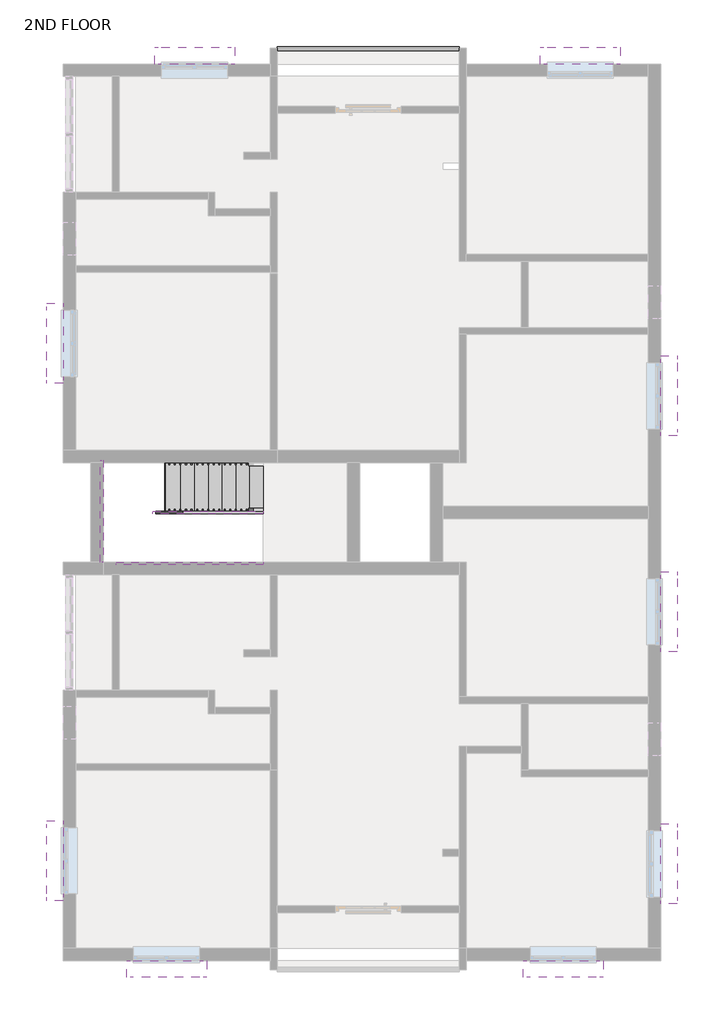
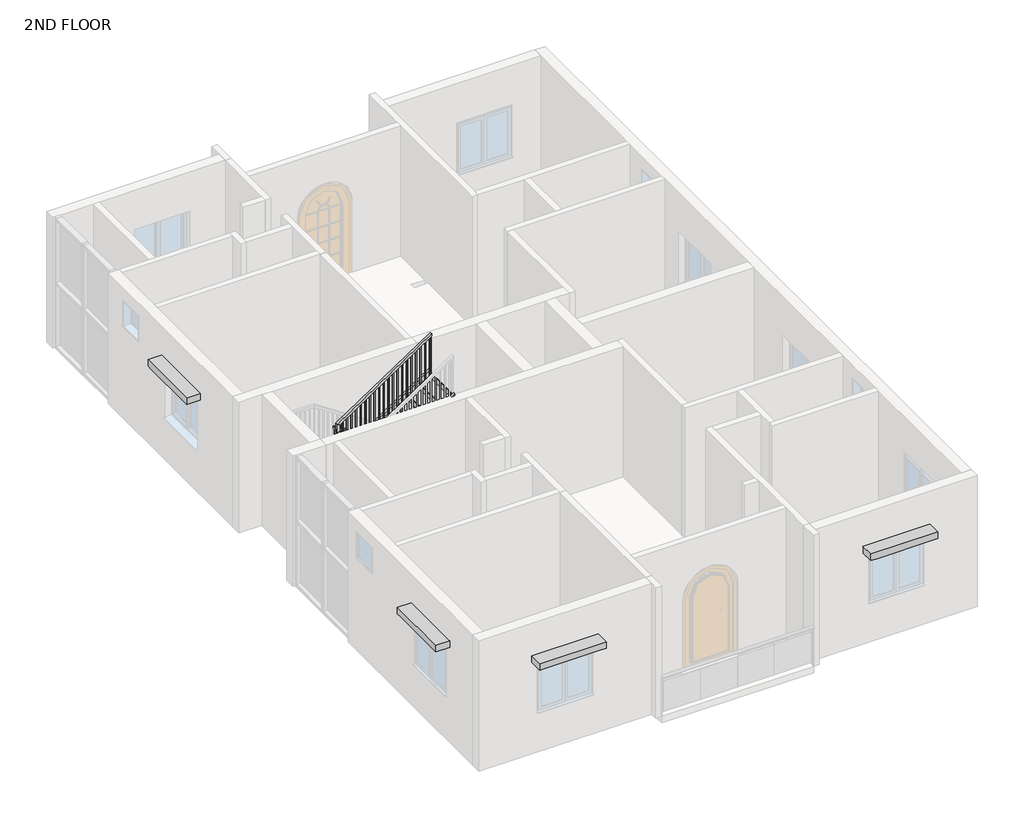
# One storey, part 4 of 4: 9 proxies, 5 members, 2 railings, 1 stair flight.
"""IFC4 building model written with IfcOpenShell, lengths in millimetres."""

from ifc_helpers import new_model, si_unit, point, frame, origin, place, context, project, spatial, polyline, ellipse_curve, trimmed, outline, extrude, faceted_brep, transform, mapped, element, save
from ifc_brep_helpers import plane_surface, extruded_surface, advanced_brep
from components import generic_models_11_generic_models_11_d301a5e8, generic_models_21_generic_models_21_87948dc1, generic_models_36_generic_models_36_9c63594f, generic_models_1_generic_models_1_fbb7ad13, stair_flight_417d3b76

model = new_model("IFC4")

# Units and contexts
model_context = context("Model", 3, world=origin())
ifc_project = project(units=[si_unit("LENGTHUNIT", "METRE", prefix="MILLI")], contexts=[model_context])

# Site, building, storey
site = spatial("IfcSite", under=ifc_project)
building = spatial("IfcBuilding", under=site)
storey = spatial("IfcBuildingStorey", under=building, Name="2ND FLOOR", Elevation=9144.0)

# Proxies
placement = place(None, origin())
generic_models_11_generic_models_11_shape = generic_models_11_generic_models_11_d301a5e8(model_context)
element("IfcBuildingElementProxy", 1, Name="Generic Models 15 : Generic Models 11", ObjectType="Generic Models 15 : Generic Models 11", at=placement, inside=storey, context=model_context, shape_type="MappedRepresentation", body=[
    mapped(generic_models_11_generic_models_11_shape, transform((0.0, 0.0, -6096.0), x_axis=(1.0, 0.0, 0.0), y_axis=(0.0, 1.0, 0.0), z_axis=(0.0, 0.0, 1.0))),
])
element("IfcBuildingElementProxy", 2, Name="Generic Models 16 : Generic Models 11", ObjectType="Generic Models 16 : Generic Models 11", at=placement, inside=storey, context=model_context, shape_type="MappedRepresentation", body=[
    mapped(generic_models_11_generic_models_11_shape, transform((-7101.0359618, 0.0, -6096.0), x_axis=(1.0, 0.0, 0.0), y_axis=(0.0, 1.0, 0.0), z_axis=(0.0, 0.0, 1.0))),
])
generic_models_21_generic_models_21_shape = generic_models_21_generic_models_21_87948dc1(model_context)
element("IfcBuildingElementProxy", 3, Name="Generic Models 27 : Generic Models 21", ObjectType="Generic Models 27 : Generic Models 21", at=placement, inside=storey, context=model_context, shape_type="MappedRepresentation", body=[
    mapped(generic_models_21_generic_models_21_shape, transform((0.0, 0.0, -6096.0), x_axis=(1.0, 0.0, 0.0), y_axis=(0.0, 1.0, 0.0), z_axis=(0.0, 0.0, 1.0))),
])
element("IfcBuildingElementProxy", 4, Name="Generic Models 28 : Generic Models 21", ObjectType="Generic Models 28 : Generic Models 21", at=placement, inside=storey, context=model_context, shape_type="MappedRepresentation", body=[
    mapped(generic_models_21_generic_models_21_shape, transform((0.0, 4641.85, -6181.6), x_axis=(1.0, 0.0, 0.0), y_axis=(0.0, 1.0, 0.0), z_axis=(0.0, 0.0, 1.0))),
])
element("IfcBuildingElementProxy", 5, Name="Generic Models 29 : Generic Models 21", ObjectType="Generic Models 29 : Generic Models 21", at=placement, inside=storey, context=model_context, shape_type="MappedRepresentation", body=[
    mapped(generic_models_21_generic_models_21_shape, transform((0.0, 8616.95, -6181.6), x_axis=(1.0, 0.0, 0.0), y_axis=(0.0, 1.0, 0.0), z_axis=(0.0, 0.0, 1.0))),
])
generic_models_36_generic_models_36_shape = generic_models_36_generic_models_36_9c63594f(model_context)
element("IfcBuildingElementProxy", 6, Name="Generic Models 40 : Generic Models 36", ObjectType="Generic Models 40 : Generic Models 36", at=placement, inside=storey, context=model_context, shape_type="MappedRepresentation", body=[
    mapped(generic_models_36_generic_models_36_shape, transform((0.0, 0.0, -6096.0), x_axis=(1.0, 0.0, 0.0), y_axis=(0.0, 1.0, 0.0), z_axis=(0.0, 0.0, 1.0))),
])
element("IfcBuildingElementProxy", 7, Name="Generic Models 41 : Generic Models 36", ObjectType="Generic Models 41 : Generic Models 36", at=placement, inside=storey, context=model_context, shape_type="MappedRepresentation", body=[
    mapped(generic_models_36_generic_models_36_shape, transform((0.0, -9525.0, -6096.0), x_axis=(1.0, 0.0, 0.0), y_axis=(0.0, 1.0, 0.0), z_axis=(0.0, 0.0, 1.0))),
])
generic_models_1_generic_models_1_shape = generic_models_1_generic_models_1_fbb7ad13(model_context)
element("IfcBuildingElementProxy", 8, Name="Generic Models 5 : Generic Models 1", ObjectType="Generic Models 5 : Generic Models 1", at=placement, inside=storey, context=model_context, shape_type="MappedRepresentation", body=[
    mapped(generic_models_1_generic_models_1_shape, transform((0.0, 0.0, -6096.0), x_axis=(1.0, 0.0, 0.0), y_axis=(0.0, 1.0, 0.0), z_axis=(0.0, 0.0, 1.0))),
])
element("IfcBuildingElementProxy", 9, Name="Generic Models 6 : Generic Models 1", ObjectType="Generic Models 6 : Generic Models 1", at=placement, inside=storey, context=model_context, shape_type="MappedRepresentation", body=[
    mapped(generic_models_1_generic_models_1_shape, transform((7304.0875, 0.0, -6096.0), x_axis=(1.0, 0.0, 0.0), y_axis=(0.0, 1.0, 0.0), z_axis=(0.0, 0.0, 1.0))),
])

# Members
element("IfcMember", 10, ObjectType="Stringer - 2\" Width", at=placement, inside=storey, context=model_context, shape_type="SweptSolid", body=[
    extrude(outline(polyline([(9144.0, -2748.0012202), (9362.0398409, -2748.0012202), (10682.8398409, -4729.2012202), (10316.5158313, -4729.2012202), (9144.0, -2970.4274732), (9144.0, -2748.0012202)])), frame((0.0, 4990.8309003, 0.0), z_axis=(0.0, 1.0, 0.0), x_axis=(0.0, 0.0, 1.0)), (0.0, 0.0, 1.0), 50.8),
])
element("IfcMember", 11, ObjectType="Stringer - 2\" Width", at=placement, inside=storey, context=model_context, shape_type="SweptSolid", body=[
    extrude(outline(polyline([(10886.0398409, -4780.0012202), (10519.7158313, -4780.0012202), (11874.382498, -2748.0012202), (12240.7065076, -2748.0012202), (10886.0398409, -4780.0012202)])), frame((0.0, 4990.8309003, 0.0), z_axis=(0.0, 1.0, 0.0), x_axis=(0.0, 0.0, 1.0)), (0.0, 0.0, 1.0), 50.8),
])
element("IfcMember", 12, ObjectType="Stringer - 2\" Width", at=placement, inside=storey, context=model_context, shape_type="SweptSolid", body=[
    extrude(outline(polyline([(9144.0, -2748.0012202), (9362.0398409, -2748.0012202), (10744.2, -4821.2414588), (10744.2, -5370.7274732), (9144.0, -2970.4274732), (9144.0, -2748.0012202)])), frame((0.0, 5930.6309003, 0.0), z_axis=(0.0, 1.0, 0.0), x_axis=(0.0, 0.0, 1.0)), (0.0, 0.0, 1.0), 50.8),
])
element("IfcMember", 13, ObjectType="Stringer - 2\" Width", at=placement, inside=storey, context=model_context, shape_type="SweptSolid", body=[
    extrude(outline(polyline([(-5745.2012202, 5981.4309003), (-5694.4012202, 5981.4309003), (-5694.4012202, 4101.8309003), (-5745.2012202, 4101.8309003), (-5745.2012202, 5981.4309003)])), frame((0.0, 0.0, 10439.4), z_axis=(0.0, 0.0, 1.0), x_axis=(1.0, 0.0, 0.0)), (0.0, 0.0, 1.0), 304.8),
])
element("IfcMember", 14, ObjectType="Stringer - 2\" Width", at=placement, inside=storey, context=model_context, shape_type="SweptSolid", body=[
    extrude(outline(polyline([(10439.4, -4900.4749672), (11874.382498, -2748.0012202), (12240.7065076, -2748.0012202), (10439.4, -5449.9609815), (10439.4, -4900.4749672)])), frame((0.0, 4051.0309003, 0.0), z_axis=(0.0, 1.0, 0.0), x_axis=(0.0, 0.0, 1.0)), (0.0, 0.0, 1.0), 50.8),
])

# Railings
element("IfcRailing", 15, ObjectType="Glass Panel - Bottom Fill 2", at=placement, inside=storey, context=model_context, shape_type="SolidModel", body=[
    advanced_brep(
    [(-2494.0012202, 13593.7910566, 10058.4), (-2494.0012202, 13517.5910566, 10058.4), (858.7987798, 13593.7910566, 10058.4), (858.7987798, 13517.5910566, 10058.4)],
    [
        (0, 1, ellipse_curve(frame((-2494.0012202, 13555.6910566, 10058.4), z_axis=(-1.0, 0.0, 0.0), x_axis=(0.0, -1.0, 0.0)), 38.1, 28.575)),
        (1, 0, ellipse_curve(frame((-2494.0012202, 13555.6910566, 10058.4), z_axis=(-1.0, 0.0, 0.0), x_axis=(0.0, -1.0, 0.0)), 38.1, 28.575)),
        (2, 3, ellipse_curve(frame((858.7987798, 13555.6910566, 10058.4), z_axis=(1.0, 0.0, 0.0), x_axis=(0.0, -1.0, 0.0)), 38.1, 28.575)),
        (3, 2, ellipse_curve(frame((858.7987798, 13555.6910566, 10058.4), z_axis=(1.0, 0.0, 0.0), x_axis=(0.0, -1.0, 0.0)), 38.1, 28.575)),
        (0, 2),
        (3, 1),
    ],
    [
        plane_surface(frame((-2494.0012202, 13555.6910566, 10058.4), z_axis=(-1.0, 0.0, 0.0), x_axis=(0.0, 1.0, 0.0))),
        plane_surface(frame((858.7987798, 13555.6910566, 10058.4), z_axis=(1.0, 0.0, 0.0), x_axis=(0.0, 1.0, 0.0))),
        extruded_surface(trimmed(ellipse_curve(frame((858.7987798, 13555.6910566, 10058.4), z_axis=(-1.0, 0.0, 0.0), x_axis=(0.0, -1.0, 0.0)), 38.1, 28.575), [point((858.7987798, 13593.7910566, 10058.4))], [point((858.7987798, 13517.5910566, 10058.4))], True, "CARTESIAN"), (-3352.7999999999997, 0.0, 0.0), 3352.7999999999997),
        extruded_surface(trimmed(ellipse_curve(frame((858.7987798, 13555.6910566, 10058.4), z_axis=(-1.0, 0.0, 0.0), x_axis=(0.0, -1.0, 0.0)), 38.1, 28.575), [point((858.7987798, 13517.5910566, 10058.4))], [point((858.7987798, 13593.7910566, 10058.4))], True, "CARTESIAN"), (-3352.7999999999997, 0.0, 0.0), 3352.7999999999997),
    ],
    [
        (0, [[1, 2]]),
        (1, [[3, 4]]),
        (2, [[-1, 5, -4, 6]]),
        (3, [[-2, -6, -3, -5]]),
    ],
),
    extrude(outline(polyline([(-4.8012202, 13562.2262136), (807.9987798, 13562.2262136), (807.9987798, 13555.8762136), (-4.8012202, 13555.8762136), (-4.8012202, 13562.2262136)])), frame((0.0, 0.0, 9245.6), z_axis=(0.0, 0.0, 1.0), x_axis=(1.0, 0.0, 0.0)), (0.0, 0.0, 1.0), 711.2),
    extrude(outline(polyline([(-817.6012202, 13562.2262136), (-4.8012202, 13562.2262136), (-4.8012202, 13555.8762136), (-817.6012202, 13555.8762136), (-817.6012202, 13562.2262136)])), frame((0.0, 0.0, 9245.6), z_axis=(0.0, 0.0, 1.0), x_axis=(1.0, 0.0, 0.0)), (0.0, 0.0, 1.0), 711.2),
    extrude(outline(polyline([(-1630.4012202, 13562.2262136), (-817.6012202, 13562.2262136), (-817.6012202, 13555.8762136), (-1630.4012202, 13555.8762136), (-1630.4012202, 13562.2262136)])), frame((0.0, 0.0, 9245.6), z_axis=(0.0, 0.0, 1.0), x_axis=(1.0, 0.0, 0.0)), (0.0, 0.0, 1.0), 711.2),
    extrude(outline(polyline([(-2443.2012202, 13562.2262136), (-1630.4012202, 13562.2262136), (-1630.4012202, 13555.8762136), (-2443.2012202, 13555.8762136), (-2443.2012202, 13562.2262136)])), frame((0.0, 0.0, 9245.6), z_axis=(0.0, 0.0, 1.0), x_axis=(1.0, 0.0, 0.0)), (0.0, 0.0, 1.0), 711.2),
    extrude(outline(polyline([(846.0987798, 13546.1660566), (846.0987798, 13565.2160566), (865.1487798, 13565.2160566), (865.1487798, 13546.1660566), (846.0987798, 13546.1660566)])), frame((0.0, 0.0, 9144.0), z_axis=(0.0, 0.0, 1.0), x_axis=(1.0, 0.0, 0.0)), (0.0, 0.0, 1.0), 885.825),
    extrude(outline(polyline([(-2500.3512202, 13546.1660566), (-2500.3512202, 13565.2160566), (-2481.3012202, 13565.2160566), (-2481.3012202, 13546.1660566), (-2500.3512202, 13546.1660566)])), frame((0.0, 0.0, 9144.0), z_axis=(0.0, 0.0, 1.0), x_axis=(1.0, 0.0, 0.0)), (0.0, 0.0, 1.0), 885.825),
])
element("IfcRailing", 16, ObjectType="Handrail - Rectangular", at=placement, inside=storey, context=model_context, shape_type="SolidModel", body=[
    faceted_brep([(-2748.0012202, 5041.6309003, 10227.7333333), (-2748.0012202, 5041.6309003, 10166.6793317), (-2748.0012202, 5092.4309003, 10166.6793317), (-2748.0012202, 5092.4309003, 10227.7333333), (-4703.8012202, 5041.6309003, 11531.6), (-4754.6012202, 5041.6309003, 11504.4126651), (-4754.6012202, 5092.4309003, 11504.4126651), (-4703.8012202, 5092.4309003, 11531.6), (-4703.8012202, 5041.6309003, 11582.4), (-4754.6012202, 5041.6309003, 11531.6), (-4754.6012202, 5092.4309003, 11531.6), (-4703.8012202, 5092.4309003, 11582.4), (-4780.0012202, 5041.6309003, 11582.4), (-4780.0012202, 5041.6309003, 11531.6), (-4830.8012202, 5092.4309003, 11531.6), (-4830.8012202, 5092.4309003, 11582.4), (-4780.0012202, 4990.8309003, 11582.4), (-4830.8012202, 4990.8309003, 11582.4), (-4830.8012202, 4940.0309003, 11531.6), (-4780.0012202, 4940.0309003, 11531.6)], [[[0, 1, 2, 3]], [[1, 0, 4, 5]], [[2, 1, 5, 6]], [[3, 2, 6, 7]], [[0, 3, 7, 4]], [[5, 4, 8, 9]], [[6, 5, 9, 10]], [[7, 6, 10, 11]], [[4, 7, 11, 8]], [[9, 8, 12, 13]], [[10, 9, 13, 14]], [[11, 10, 14, 15]], [[8, 11, 15, 12]], [[16, 17, 18, 19]], [[13, 12, 16, 19]], [[14, 13, 19, 18]], [[15, 14, 18, 17]], [[12, 15, 17, 16]]]),
    faceted_brep([(-4780.0012202, 4990.8309003, 11582.4), (-4780.0012202, 4940.0309003, 11531.6), (-4830.8012202, 4940.0309003, 11531.6), (-4830.8012202, 4990.8309003, 11582.4), (-4780.0012202, 4990.8309003, 11690.6793317), (-4830.8012202, 4990.8309003, 11717.8666667), (-4830.8012202, 4940.0309003, 11717.8666667), (-4780.0012202, 4940.0309003, 11690.6793317)], [[[0, 1, 2, 3]], [[4, 5, 6, 7]], [[1, 0, 4, 7]], [[2, 1, 7, 6]], [[3, 2, 6, 5]], [[0, 3, 5, 4]]]),
    faceted_brep([(-4830.8012202, 4990.8309003, 11717.8666667), (-4780.0012202, 4990.8309003, 11690.6793317), (-4780.0012202, 4940.0309003, 11690.6793317), (-4830.8012202, 4940.0309003, 11717.8666667), (-2748.0012202, 4990.8309003, 13106.4), (-2748.0012202, 4940.0309003, 13106.4), (-2748.0012202, 4940.0309003, 13045.3459984), (-2748.0012202, 4990.8309003, 13045.3459984)], [[[0, 1, 2, 3]], [[4, 5, 6, 7]], [[1, 0, 4, 7]], [[2, 1, 7, 6]], [[3, 2, 6, 5]], [[0, 3, 5, 4]]]),
    extrude(outline(polyline([(13022.0626651, -2782.9262202), (12022.6666667, -2782.9262202), (12022.6666667, -2763.8762202), (13034.7626651, -2763.8762202), (13022.0626651, -2782.9262202)])), frame((0.0, 4955.9059003, 0.0), z_axis=(0.0, 1.0, 0.0), x_axis=(0.0, 0.0, 1.0)), (0.0, 0.0, 1.0), 19.05),
    extrude(outline(polyline([(12954.3293317, -2884.5262202), (12022.6666667, -2884.5262202), (12022.6666667, -2865.4762202), (12967.0293317, -2865.4762202), (12954.3293317, -2884.5262202)])), frame((0.0, 4955.9059003, 0.0), z_axis=(0.0, 1.0, 0.0), x_axis=(0.0, 0.0, 1.0)), (0.0, 0.0, 1.0), 19.05),
    extrude(outline(polyline([(12886.5959984, -2986.1262202), (12022.6666667, -2986.1262202), (12022.6666667, -2967.0762202), (12899.2959984, -2967.0762202), (12886.5959984, -2986.1262202)])), frame((0.0, 4955.9059003, 0.0), z_axis=(0.0, 1.0, 0.0), x_axis=(0.0, 0.0, 1.0)), (0.0, 0.0, 1.0), 19.05),
    extrude(outline(polyline([(12818.8626651, -3087.7262202), (11853.3333333, -3087.7262202), (11853.3333333, -3068.6762202), (12831.5626651, -3068.6762202), (12818.8626651, -3087.7262202)])), frame((0.0, 4955.9059003, 0.0), z_axis=(0.0, 1.0, 0.0), x_axis=(0.0, 0.0, 1.0)), (0.0, 0.0, 1.0), 19.05),
    extrude(outline(polyline([(12751.1293317, -3189.3262202), (11853.3333333, -3189.3262202), (11853.3333333, -3170.2762202), (12763.8293317, -3170.2762202), (12751.1293317, -3189.3262202)])), frame((0.0, 4955.9059003, 0.0), z_axis=(0.0, 1.0, 0.0), x_axis=(0.0, 0.0, 1.0)), (0.0, 0.0, 1.0), 19.05),
    extrude(outline(polyline([(12683.3959984, -3290.9262202), (11684.0, -3290.9262202), (11684.0, -3271.8762202), (12696.0959984, -3271.8762202), (12683.3959984, -3290.9262202)])), frame((0.0, 4955.9059003, 0.0), z_axis=(0.0, 1.0, 0.0), x_axis=(0.0, 0.0, 1.0)), (0.0, 0.0, 1.0), 19.05),
    extrude(outline(polyline([(12615.6626651, -3392.5262202), (11684.0, -3392.5262202), (11684.0, -3373.4762202), (12628.3626651, -3373.4762202), (12615.6626651, -3392.5262202)])), frame((0.0, 4955.9059003, 0.0), z_axis=(0.0, 1.0, 0.0), x_axis=(0.0, 0.0, 1.0)), (0.0, 0.0, 1.0), 19.05),
    extrude(outline(polyline([(12547.9293317, -3494.1262202), (11684.0, -3494.1262202), (11684.0, -3475.0762202), (12560.6293317, -3475.0762202), (12547.9293317, -3494.1262202)])), frame((0.0, 4955.9059003, 0.0), z_axis=(0.0, 1.0, 0.0), x_axis=(0.0, 0.0, 1.0)), (0.0, 0.0, 1.0), 19.05),
    extrude(outline(polyline([(12480.1959984, -3595.7262202), (11514.6666667, -3595.7262202), (11514.6666667, -3576.6762202), (12492.8959984, -3576.6762202), (12480.1959984, -3595.7262202)])), frame((0.0, 4955.9059003, 0.0), z_axis=(0.0, 1.0, 0.0), x_axis=(0.0, 0.0, 1.0)), (0.0, 0.0, 1.0), 19.05),
    extrude(outline(polyline([(12412.4626651, -3697.3262202), (11514.6666667, -3697.3262202), (11514.6666667, -3678.2762202), (12425.1626651, -3678.2762202), (12412.4626651, -3697.3262202)])), frame((0.0, 4955.9059003, 0.0), z_axis=(0.0, 1.0, 0.0), x_axis=(0.0, 0.0, 1.0)), (0.0, 0.0, 1.0), 19.05),
    extrude(outline(polyline([(12344.7293317, -3798.9262202), (11345.3333333, -3798.9262202), (11345.3333333, -3779.8762202), (12357.4293317, -3779.8762202), (12344.7293317, -3798.9262202)])), frame((0.0, 4955.9059003, 0.0), z_axis=(0.0, 1.0, 0.0), x_axis=(0.0, 0.0, 1.0)), (0.0, 0.0, 1.0), 19.05),
    extrude(outline(polyline([(12276.9959984, -3900.5262202), (11345.3333333, -3900.5262202), (11345.3333333, -3881.4762202), (12289.6959984, -3881.4762202), (12276.9959984, -3900.5262202)])), frame((0.0, 4955.9059003, 0.0), z_axis=(0.0, 1.0, 0.0), x_axis=(0.0, 0.0, 1.0)), (0.0, 0.0, 1.0), 19.05),
    extrude(outline(polyline([(12209.2626651, -4002.1262202), (11345.3333333, -4002.1262202), (11345.3333333, -3983.0762202), (12221.9626651, -3983.0762202), (12209.2626651, -4002.1262202)])), frame((0.0, 4955.9059003, 0.0), z_axis=(0.0, 1.0, 0.0), x_axis=(0.0, 0.0, 1.0)), (0.0, 0.0, 1.0), 19.05),
    extrude(outline(polyline([(12141.5293317, -4103.7262202), (11176.0, -4103.7262202), (11176.0, -4084.6762202), (12154.2293317, -4084.6762202), (12141.5293317, -4103.7262202)])), frame((0.0, 4955.9059003, 0.0), z_axis=(0.0, 1.0, 0.0), x_axis=(0.0, 0.0, 1.0)), (0.0, 0.0, 1.0), 19.05),
    extrude(outline(polyline([(12073.7959984, -4205.3262202), (11176.0, -4205.3262202), (11176.0, -4186.2762202), (12086.4959984, -4186.2762202), (12073.7959984, -4205.3262202)])), frame((0.0, 4955.9059003, 0.0), z_axis=(0.0, 1.0, 0.0), x_axis=(0.0, 0.0, 1.0)), (0.0, 0.0, 1.0), 19.05),
    extrude(outline(polyline([(12006.0626651, -4306.9262202), (11006.6666667, -4306.9262202), (11006.6666667, -4287.8762202), (12018.7626651, -4287.8762202), (12006.0626651, -4306.9262202)])), frame((0.0, 4955.9059003, 0.0), z_axis=(0.0, 1.0, 0.0), x_axis=(0.0, 0.0, 1.0)), (0.0, 0.0, 1.0), 19.05),
    extrude(outline(polyline([(11938.3293317, -4408.5262202), (11006.6666667, -4408.5262202), (11006.6666667, -4389.4762202), (11951.0293317, -4389.4762202), (11938.3293317, -4408.5262202)])), frame((0.0, 4955.9059003, 0.0), z_axis=(0.0, 1.0, 0.0), x_axis=(0.0, 0.0, 1.0)), (0.0, 0.0, 1.0), 19.05),
    extrude(outline(polyline([(11870.5959984, -4510.1262202), (11006.6666667, -4510.1262202), (11006.6666667, -4491.0762202), (11883.2959984, -4491.0762202), (11870.5959984, -4510.1262202)])), frame((0.0, 4955.9059003, 0.0), z_axis=(0.0, 1.0, 0.0), x_axis=(0.0, 0.0, 1.0)), (0.0, 0.0, 1.0), 19.05),
    extrude(outline(polyline([(11802.8626651, -4611.7262202), (10837.3333333, -4611.7262202), (10837.3333333, -4592.6762202), (11815.5626651, -4592.6762202), (11802.8626651, -4611.7262202)])), frame((0.0, 4955.9059003, 0.0), z_axis=(0.0, 1.0, 0.0), x_axis=(0.0, 0.0, 1.0)), (0.0, 0.0, 1.0), 19.05),
    extrude(outline(polyline([(11735.1293317, -4713.3262202), (10837.3333333, -4713.3262202), (10837.3333333, -4694.2762202), (11747.8293317, -4694.2762202), (11735.1293317, -4713.3262202)])), frame((0.0, 4955.9059003, 0.0), z_axis=(0.0, 1.0, 0.0), x_axis=(0.0, 0.0, 1.0)), (0.0, 0.0, 1.0), 19.05),
    extrude(outline(polyline([(-4770.4762202, 5057.5059003), (-4789.5262202, 5057.5059003), (-4789.5262202, 5076.5559003), (-4770.4762202, 5076.5559003), (-4770.4762202, 5057.5059003)])), frame((0.0, 0.0, 10668.0), z_axis=(0.0, 0.0, 1.0), x_axis=(1.0, 0.0, 0.0)), (0.0, 0.0, 1.0), 863.6),
    extrude(outline(polyline([(11459.9626651, -4687.9262202), (10498.6666667, -4687.9262202), (10498.6666667, -4668.8762202), (11447.2626651, -4668.8762202), (11459.9626651, -4687.9262202)])), frame((0.0, 5057.5059003, 0.0), z_axis=(0.0, 1.0, 0.0), x_axis=(0.0, 0.0, 1.0)), (0.0, 0.0, 1.0), 19.05),
    extrude(outline(polyline([(11392.2293317, -4586.3262202), (10498.6666667, -4586.3262202), (10498.6666667, -4567.2762202), (11379.5293317, -4567.2762202), (11392.2293317, -4586.3262202)])), frame((0.0, 5057.5059003, 0.0), z_axis=(0.0, 1.0, 0.0), x_axis=(0.0, 0.0, 1.0)), (0.0, 0.0, 1.0), 19.05),
    extrude(outline(polyline([(11324.4959984, -4484.7262202), (10329.3333333, -4484.7262202), (10329.3333333, -4465.6762202), (11311.7959984, -4465.6762202), (11324.4959984, -4484.7262202)])), frame((0.0, 5057.5059003, 0.0), z_axis=(0.0, 1.0, 0.0), x_axis=(0.0, 0.0, 1.0)), (0.0, 0.0, 1.0), 19.05),
    extrude(outline(polyline([(11256.7626651, -4383.1262202), (10329.3333333, -4383.1262202), (10329.3333333, -4364.0762202), (11244.0626651, -4364.0762202), (11256.7626651, -4383.1262202)])), frame((0.0, 5057.5059003, 0.0), z_axis=(0.0, 1.0, 0.0), x_axis=(0.0, 0.0, 1.0)), (0.0, 0.0, 1.0), 19.05),
    extrude(outline(polyline([(11189.0293317, -4281.5262202), (10329.3333333, -4281.5262202), (10329.3333333, -4262.4762202), (11176.3293317, -4262.4762202), (11189.0293317, -4281.5262202)])), frame((0.0, 5057.5059003, 0.0), z_axis=(0.0, 1.0, 0.0), x_axis=(0.0, 0.0, 1.0)), (0.0, 0.0, 1.0), 19.05),
    extrude(outline(polyline([(11121.2959984, -4179.9262202), (10160.0, -4179.9262202), (10160.0, -4160.8762202), (11108.5959984, -4160.8762202), (11121.2959984, -4179.9262202)])), frame((0.0, 5057.5059003, 0.0), z_axis=(0.0, 1.0, 0.0), x_axis=(0.0, 0.0, 1.0)), (0.0, 0.0, 1.0), 19.05),
    extrude(outline(polyline([(11053.5626651, -4078.3262202), (10160.0, -4078.3262202), (10160.0, -4059.2762202), (11040.8626651, -4059.2762202), (11053.5626651, -4078.3262202)])), frame((0.0, 5057.5059003, 0.0), z_axis=(0.0, 1.0, 0.0), x_axis=(0.0, 0.0, 1.0)), (0.0, 0.0, 1.0), 19.05),
    extrude(outline(polyline([(10985.8293317, -3976.7262202), (9990.6666667, -3976.7262202), (9990.6666667, -3957.6762202), (10973.1293317, -3957.6762202), (10985.8293317, -3976.7262202)])), frame((0.0, 5057.5059003, 0.0), z_axis=(0.0, 1.0, 0.0), x_axis=(0.0, 0.0, 1.0)), (0.0, 0.0, 1.0), 19.05),
    extrude(outline(polyline([(10918.0959984, -3875.1262202), (9990.6666667, -3875.1262202), (9990.6666667, -3856.0762202), (10905.3959984, -3856.0762202), (10918.0959984, -3875.1262202)])), frame((0.0, 5057.5059003, 0.0), z_axis=(0.0, 1.0, 0.0), x_axis=(0.0, 0.0, 1.0)), (0.0, 0.0, 1.0), 19.05),
    extrude(outline(polyline([(10850.3626651, -3773.5262202), (9990.6666667, -3773.5262202), (9990.6666667, -3754.4762202), (10837.6626651, -3754.4762202), (10850.3626651, -3773.5262202)])), frame((0.0, 5057.5059003, 0.0), z_axis=(0.0, 1.0, 0.0), x_axis=(0.0, 0.0, 1.0)), (0.0, 0.0, 1.0), 19.05),
    extrude(outline(polyline([(10782.6293317, -3671.9262202), (9821.3333333, -3671.9262202), (9821.3333333, -3652.8762202), (10769.9293317, -3652.8762202), (10782.6293317, -3671.9262202)])), frame((0.0, 5057.5059003, 0.0), z_axis=(0.0, 1.0, 0.0), x_axis=(0.0, 0.0, 1.0)), (0.0, 0.0, 1.0), 19.05),
    extrude(outline(polyline([(10714.8959984, -3570.3262202), (9821.3333333, -3570.3262202), (9821.3333333, -3551.2762202), (10702.1959984, -3551.2762202), (10714.8959984, -3570.3262202)])), frame((0.0, 5057.5059003, 0.0), z_axis=(0.0, 1.0, 0.0), x_axis=(0.0, 0.0, 1.0)), (0.0, 0.0, 1.0), 19.05),
    extrude(outline(polyline([(10647.1626651, -3468.7262202), (9652.0, -3468.7262202), (9652.0, -3449.6762202), (10634.4626651, -3449.6762202), (10647.1626651, -3468.7262202)])), frame((0.0, 5057.5059003, 0.0), z_axis=(0.0, 1.0, 0.0), x_axis=(0.0, 0.0, 1.0)), (0.0, 0.0, 1.0), 19.05),
    extrude(outline(polyline([(10579.4293317, -3367.1262202), (9652.0, -3367.1262202), (9652.0, -3348.0762202), (10566.7293317, -3348.0762202), (10579.4293317, -3367.1262202)])), frame((0.0, 5057.5059003, 0.0), z_axis=(0.0, 1.0, 0.0), x_axis=(0.0, 0.0, 1.0)), (0.0, 0.0, 1.0), 19.05),
    extrude(outline(polyline([(10511.6959984, -3265.5262202), (9652.0, -3265.5262202), (9652.0, -3246.4762202), (10498.9959984, -3246.4762202), (10511.6959984, -3265.5262202)])), frame((0.0, 5057.5059003, 0.0), z_axis=(0.0, 1.0, 0.0), x_axis=(0.0, 0.0, 1.0)), (0.0, 0.0, 1.0), 19.05),
    extrude(outline(polyline([(10443.9626651, -3163.9262202), (9482.6666667, -3163.9262202), (9482.6666667, -3144.8762202), (10431.2626651, -3144.8762202), (10443.9626651, -3163.9262202)])), frame((0.0, 5057.5059003, 0.0), z_axis=(0.0, 1.0, 0.0), x_axis=(0.0, 0.0, 1.0)), (0.0, 0.0, 1.0), 19.05),
    extrude(outline(polyline([(10376.2293317, -3062.3262202), (9482.6666667, -3062.3262202), (9482.6666667, -3043.2762202), (10363.5293317, -3043.2762202), (10376.2293317, -3062.3262202)])), frame((0.0, 5057.5059003, 0.0), z_axis=(0.0, 1.0, 0.0), x_axis=(0.0, 0.0, 1.0)), (0.0, 0.0, 1.0), 19.05),
    extrude(outline(polyline([(10308.4959984, -2960.7262202), (9313.3333333, -2960.7262202), (9313.3333333, -2941.6762202), (10295.7959984, -2941.6762202), (10308.4959984, -2960.7262202)])), frame((0.0, 5057.5059003, 0.0), z_axis=(0.0, 1.0, 0.0), x_axis=(0.0, 0.0, 1.0)), (0.0, 0.0, 1.0), 19.05),
    extrude(outline(polyline([(10240.7626651, -2859.1262202), (9313.3333333, -2859.1262202), (9313.3333333, -2840.0762202), (10228.0626651, -2840.0762202), (10240.7626651, -2859.1262202)])), frame((0.0, 5057.5059003, 0.0), z_axis=(0.0, 1.0, 0.0), x_axis=(0.0, 0.0, 1.0)), (0.0, 0.0, 1.0), 19.05),
    extrude(outline(polyline([(-4795.8762202, 4974.9559003), (-4795.8762202, 4955.9059003), (-4814.9262202, 4955.9059003), (-4814.9262202, 4974.9559003), (-4795.8762202, 4974.9559003)])), frame((0.0, 0.0, 10668.0), z_axis=(0.0, 0.0, 1.0), x_axis=(1.0, 0.0, 0.0)), (0.0, 0.0, 1.0), 863.6),
    extrude(outline(polyline([(-4795.8762202, 5057.5059003), (-4814.9262202, 5057.5059003), (-4814.9262202, 5076.5559003), (-4795.8762202, 5076.5559003), (-4795.8762202, 5057.5059003)])), frame((0.0, 0.0, 10668.0), z_axis=(0.0, 0.0, 1.0), x_axis=(1.0, 0.0, 0.0)), (0.0, 0.0, 1.0), 863.6),
    extrude(outline(polyline([(13032.6459984, -2767.0512202), (12022.6666667, -2767.0512202), (12022.6666667, -2748.0012202), (13045.3459984, -2748.0012202), (13032.6459984, -2767.0512202)])), frame((0.0, 4955.9059003, 0.0), z_axis=(0.0, 1.0, 0.0), x_axis=(0.0, 0.0, 1.0)), (0.0, 0.0, 1.0), 19.05),
    extrude(outline(polyline([(10179.3793317, -2767.0512202), (9313.3333333, -2767.0512202), (9313.3333333, -2748.0012202), (10166.6793317, -2748.0012202), (10179.3793317, -2767.0512202)])), frame((0.0, 5057.5059003, 0.0), z_axis=(0.0, 1.0, 0.0), x_axis=(0.0, 0.0, 1.0)), (0.0, 0.0, 1.0), 19.05),
])

# Stair flight
stair_flight_shape = stair_flight_417d3b76(model_context)
element("IfcStairFlight", 17, ObjectType="2\" Tread 1\" Nosing 1/4\" Riser", at=placement, inside=storey, context=model_context, shape_type="MappedRepresentation", body=[
    mapped(stair_flight_shape, transform((0.0, 0.0, 0.0), x_axis=(1.0, 0.0, 0.0), y_axis=(0.0, 1.0, 0.0), z_axis=(0.0, 0.0, 1.0))),
])

save(model, "model.ifc")

# Revit data of these elements
# Type "Glass Panel - Bottom Fill 2"
#   Assembly Code = "C2010400"
#   built-in parameter 1008612 = 0.0416667 (stored number, unit not read)
#   built-in parameter 1008611 = 0.0416667 (stored number, unit not read)
#   built-in parameter 1008609 = 0.333333 (stored number, unit not read)
#   built-in parameter 1008604 = 0.166667 (stored number, unit not read)
#   built-in parameter 1008603 = 0.166667 (stored number, unit not read)
#   Railing Height = 3' - 0"
#   built-in parameter 1008630 = 2
#   built-in parameter 1008610 = 2
#   built-in parameter 1008618 = Baluster - Square : 3/4"
# Type "Handrail - Rectangular"
#   Assembly Code = "C2010400"
#   built-in parameter 1008612 = 0.0416667 (stored number, unit not read)
#   built-in parameter 1008611 = 0.0416667 (stored number, unit not read)
#   built-in parameter 1008609 = 0.333333 (stored number, unit not read)
#   built-in parameter 1008604 = 0.166667 (stored number, unit not read)
#   built-in parameter 1008603 = 0.166667 (stored number, unit not read)
#   Railing Height = 3' - 0"
#   built-in parameter 1008630 = 2
#   built-in parameter 1008610 = 2
#   built-in parameter 1008618 = Baluster - Square : 3/4"
# Element 1 (IfcBuildingElementProxy, "Generic Models 15 : Generic Models 11")
#   Phase Created = New Construction
#   Materials on its faces: "white"
# Element 2 (IfcBuildingElementProxy, "Generic Models 16 : Generic Models 11")
#   Phase Created = New Construction
#   Materials on its faces: "white"
# Element 3 (IfcBuildingElementProxy, "Generic Models 27 : Generic Models 21")
#   Phase Created = New Construction
#   Materials on its faces: "white"
# Element 4 (IfcBuildingElementProxy, "Generic Models 28 : Generic Models 21")
#   Phase Created = New Construction
#   Materials on its faces: "white"
# Element 5 (IfcBuildingElementProxy, "Generic Models 29 : Generic Models 21")
#   Phase Created = New Construction
#   Materials on its faces: "white"
# Element 6 (IfcBuildingElementProxy, "Generic Models 40 : Generic Models 36")
#   Phase Created = New Construction
#   Materials on its faces: "white"
# Element 7 (IfcBuildingElementProxy, "Generic Models 41 : Generic Models 36")
#   Phase Created = New Construction
#   Materials on its faces: "white"
# Element 8 (IfcBuildingElementProxy, "Generic Models 5 : Generic Models 1")
#   Phase Created = New Construction
#   Materials on its faces: "white"
# Element 9 (IfcBuildingElementProxy, "Generic Models 6 : Generic Models 1")
#   Phase Created = New Construction
#   Materials on its faces: "white"
# Elements 10, 11, 12, 13, 14 (IfcMember, "Stringer - 2\" Width")
#   Phase Created = New Construction
# Element 15 (IfcRailing, "Glass Panel - Bottom Fill 2")
#   Phase Created = New Construction
#   Materials on its faces: "Glass"
# Element 16 (IfcRailing, "Handrail - Rectangular")
#   Phase Created = New Construction
# Element 17 (IfcStairFlight, "2\" Tread 1\" Nosing 1/4\" Riser")
#   Phase Created = New Construction
# Materials
#   "white": class "Generic", colour RGB 120 120 120, transparency 0, Cost = 0
#   "Glass": class "Glass", colour RGB 0 128 192, transparency 0.75, Description = "Soda Lime Glass", Cost = 0
